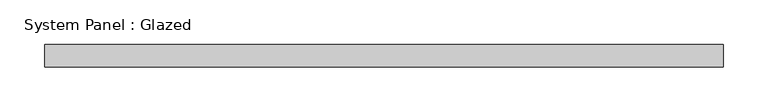
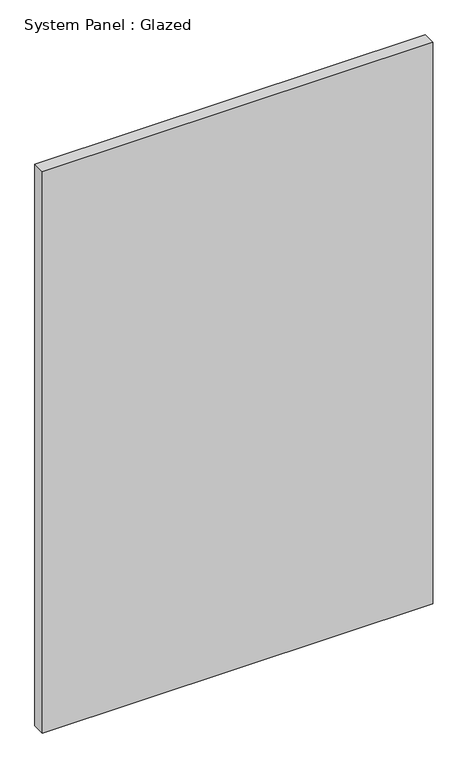
"""IFC4 building model written with IfcOpenShell, lengths in millimetres: plate geometry, System Panel : Glazed."""

from ifc_helpers import new_model, si_unit, origin, origin_with_axes, place, context, project, spatial, polyline, outline, extrude, source, transform, mapped, element, save


def system_panel_glazed_fa5755b7(model_context):
    return source(origin(), model_context, "Body", "SweptSolid", [
        extrude(outline(polyline([(380.0616098, 19.05), (-380.0616098, 19.05), (-380.0616098, 44.45), (380.0616098, 44.45), (380.0616098, 19.05)])), origin_with_axes(), (0.0, 0.0, 1.0), 1155.7),
    ])


if __name__ == "__main__":
    model = new_model("IFC4")
    model_context = context("Model", 3, world=origin())
    ifc_project = project(units=[si_unit("LENGTHUNIT", "METRE", prefix="MILLI")], contexts=[model_context])
    site = spatial("IfcSite", under=ifc_project)
    building = spatial("IfcBuilding", under=site)
    placement = place(None, origin())
    system_panel_glazed_shape = system_panel_glazed_fa5755b7(model_context)
    element("IfcPlate", 1, ObjectType="System Panel : Glazed", at=placement, inside=building, context=model_context, shape_type="MappedRepresentation", body=[
        mapped(system_panel_glazed_shape, transform((0.0, 0.0, 0.0), x_axis=(1.0, 0.0, 0.0), y_axis=(0.0, 1.0, 0.0), z_axis=(0.0, 0.0, 1.0))),
    ])
    save(model, "model.ifc")

# Revit data of these elements
# Type "System Panel : Glazed"
#   Construction Type Id = "GSP4R"
#   Analytic Construction = "1/8 in Pilkington single glazing"
#   Visual Light Transmittance = 0.9
#   Solar Heat Gain Coefficient = 0.86
#   Heat Transfer Coefficient (U) = 1.18115 BTU/(h·ft²·°F)
# Element 1 (IfcPlate, "System Panel : Glazed")
#   Materials on its faces: "Glass"
# Materials
#   "Glass": class "Glass", colour RGB 0 128 192, transparency 0.75, Description = "Soda Lime Glass", Cost = 0
